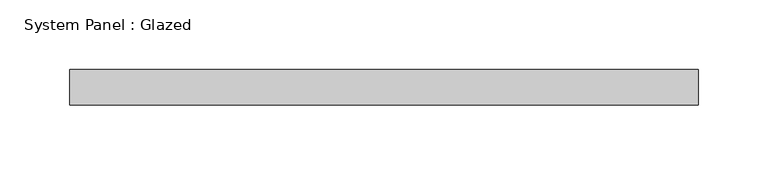
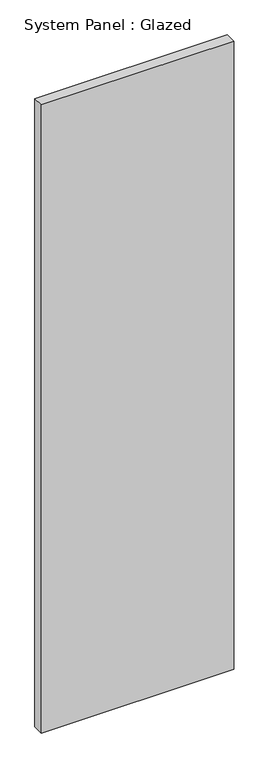
"""IFC4 building model written with IfcOpenShell, lengths in millimetres: plate geometry, System Panel : Glazed."""

from ifc_helpers import new_model, si_unit, origin, origin_with_axes, place, context, project, spatial, polyline, outline, extrude, source, transform, mapped, element, save


def system_panel_glazed_7e68e824(model_context):
    return source(origin(), model_context, "Body", "SweptSolid", [
        extrude(outline(polyline([(225.425, 19.05), (-225.425, 19.05), (-225.425, 44.45), (225.425, 44.45), (225.425, 19.05)])), origin_with_axes(), (0.0, 0.0, 1.0), 1555.0744644),
    ])


if __name__ == "__main__":
    model = new_model("IFC4")
    model_context = context("Model", 3, world=origin())
    ifc_project = project(units=[si_unit("LENGTHUNIT", "METRE", prefix="MILLI")], contexts=[model_context])
    site = spatial("IfcSite", under=ifc_project)
    building = spatial("IfcBuilding", under=site)
    placement = place(None, origin())
    system_panel_glazed_shape = system_panel_glazed_7e68e824(model_context)
    element("IfcPlate", 1, ObjectType="System Panel : Glazed", at=placement, inside=building, context=model_context, shape_type="MappedRepresentation", body=[
        mapped(system_panel_glazed_shape, transform((0.0, 0.0, 0.0), x_axis=(1.0, 0.0, 0.0), y_axis=(0.0, 1.0, 0.0), z_axis=(0.0, 0.0, 1.0))),
    ])
    save(model, "model.ifc")

# Revit data of these elements
# Type "System Panel : Glazed"
#   Construction Type Id = "GSP4R"
#   Analytic Construction = "1/8 in Pilkington single glazing"
#   Visual Light Transmittance = 0.9
#   Solar Heat Gain Coefficient = 0.86
#   Heat Transfer Coefficient (U) = 1.18115 BTU/(h·ft²·°F)
#   Define Thermal Properties by = 1
# Element 1 (IfcPlate, "System Panel : Glazed")
#   Materials on its faces: "Glass"
# Materials
#   "Glass": class "Glass", colour RGB 0 128 192, transparency 0.75, Description = "Soda Lime Glass", Cost = 0
